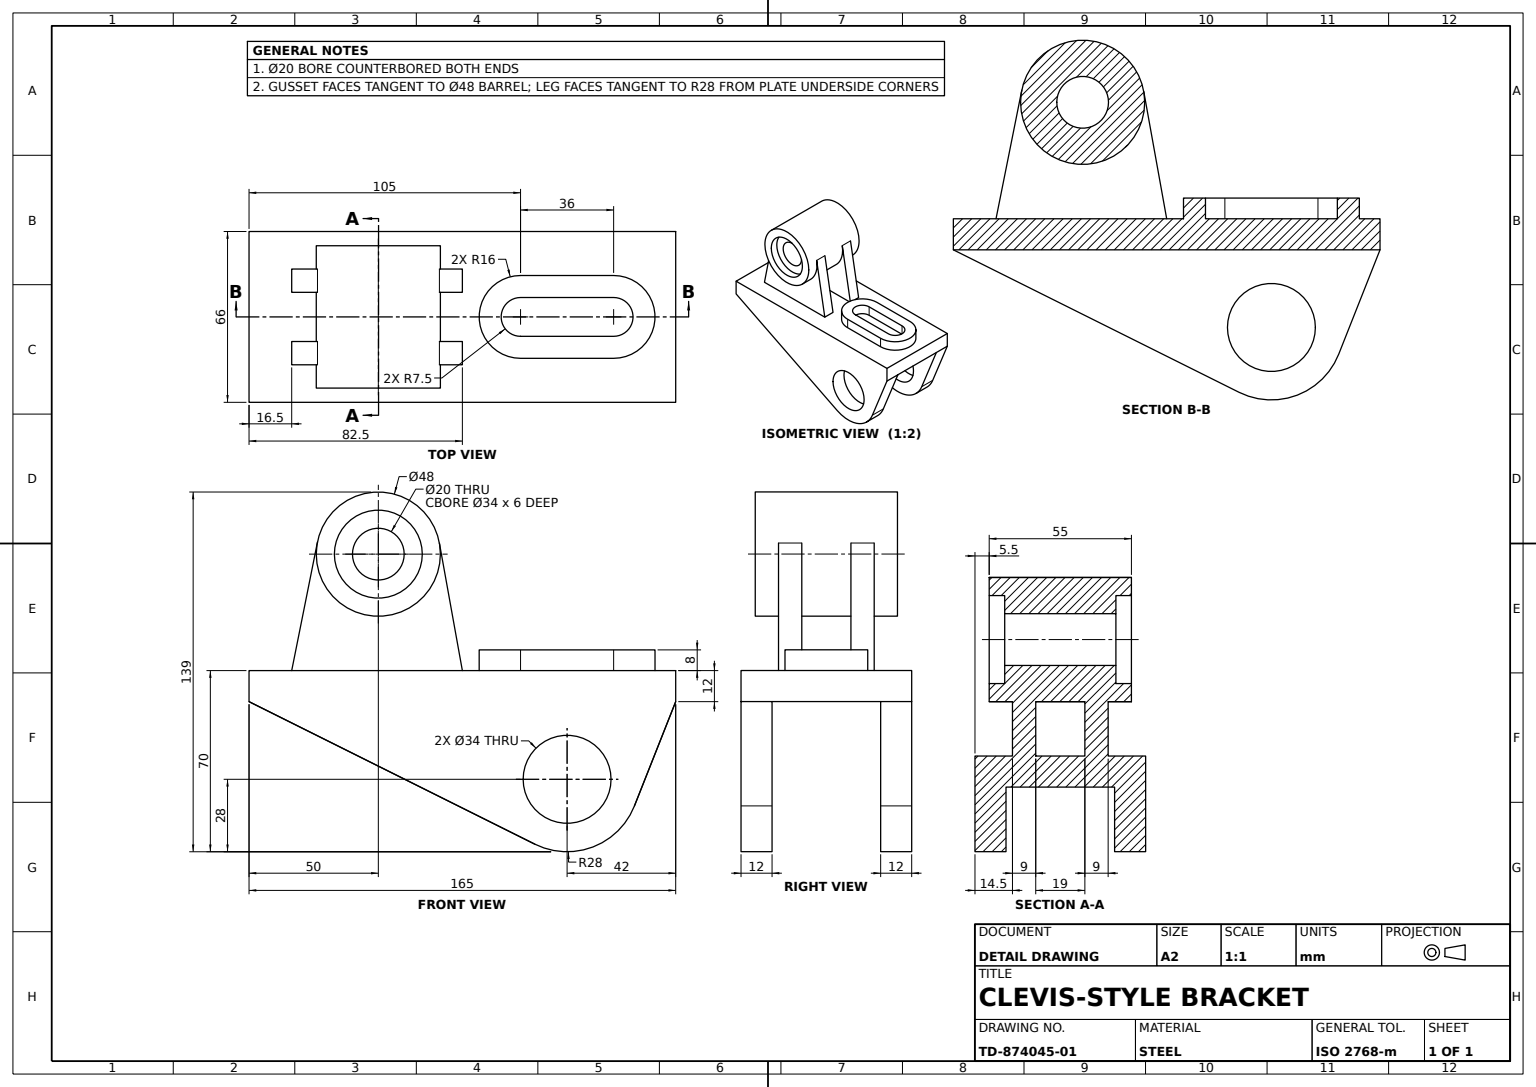
from build123d import *

# Parameters (mm, degrees)
STANCHION_PROFILE_SKETCH_R = 17
STANCHION_BODY_DEPTH       = 33
CORNER_NOTCH_SKETCH_W      = 42
CORNER_NOTCH_SKETCH_H      = 58
CORNER_NOTCH_12X12_DEPTH   = 183.247085025
SLOTTED_BOSS_DEPTH         = 8
HINGE_BARREL_SKETCH_R      = 24
HINGE_BARREL_SKETCH_R_2    = 10
HINGE_BARREL_DEPTH         = 27.5
BARREL_START               = -9
BARREL_GUSSET_DEPTH        = 9
BARREL_RECESS_SKETCH_R     = 17
BARREL_RECESS_CUT_DEPTH    = 6


with BuildPart() as part:
    # Stanchion Profile Sketch → Stanchion Body (new, symmetric)
    with BuildSketch(Plane.XY):
        with BuildLine():
            Line((0, 0), (165, 0))
            Line((165, 0), (165, -12))
            Line((165, -12), (149.032106642, -52.311615965))
            ThreePointArc((149.032106642, -52.311615965), (133.013045842, -68.148401729), (110.513423096, -67.061631974))
            Line((110.513423096, -67.061631974), (0, -12))
            Line((0, -12), (0, 0))
        make_face()
        with Locations((123, -42)):
            Circle(STANCHION_PROFILE_SKETCH_R, mode=Mode.SUBTRACT)
    extrude(amount=STANCHION_BODY_DEPTH, both=True)

    # Corner Notch Sketch → Corner Notch 12x12 (cut, through all)
    with BuildSketch(Plane(origin=(165, 0, 0), x_dir=(0, 0, -1), z_dir=(1, 0, 0))):
        with Locations((0, -41)):
            Rectangle(CORNER_NOTCH_SKETCH_W, CORNER_NOTCH_SKETCH_H)
    extrude(amount=-CORNER_NOTCH_12X12_DEPTH, mode=Mode.SUBTRACT)

    # Slotted Boss Sketch → Slotted Boss (add)
    with BuildSketch(Plane(origin=(0, 0, 0), x_dir=(1, 0, 0), z_dir=(0, 1, 0))):
        with BuildLine():
            Line((105, 16), (141, 16))
            ThreePointArc((141, 16), (157, 0), (141, -16))
            Line((141, -16), (105, -16))
            ThreePointArc((105, -16), (89, 0), (105, 16))
        make_face()
        with BuildLine():
            Line((105, 7.5), (141, 7.5))
            ThreePointArc((141, 7.5), (148.5, 0), (141, -7.5))
            Line((141, -7.5), (105, -7.5))
            ThreePointArc((105, -7.5), (97.5, 0), (105, 7.5))
        make_face(mode=Mode.SUBTRACT)
    extrude(amount=SLOTTED_BOSS_DEPTH)



with BuildPart() as body_2:
    # Hinge Barrel Sketch → Hinge Barrel (new, symmetric)
    with BuildSketch(Plane.XY):
        with Locations((50, 45)):
            Circle(HINGE_BARREL_SKETCH_R)
        with Locations((50, 45)):
            Circle(HINGE_BARREL_SKETCH_R_2, mode=Mode.SUBTRACT)
    extrude(amount=HINGE_BARREL_DEPTH, both=True)


with BuildPart() as part_1:
    add(part.part)

    add(body_2.part)  # Barrel Gusset merges body 2
    # Barrel Gusset Sketch → Barrel Gusset (add)
    with BuildSketch(Plane.XY.offset(27.5).offset(BARREL_START)):
        with BuildLine():
            Line((73.619203331, 49.258313517), (82.5, 0))
            Line((82.5, 0), (16.5, 0))
            Line((16.5, 0), (26.468315489, 49.718031802))
            ThreePointArc((26.468315489, 49.718031802), (49.766012583, 21.001140654), (73.619203331, 49.258313517))
        make_face()
    barrel_gusset = extrude(amount=-BARREL_GUSSET_DEPTH)

    # Barrel Gusset Mirror: Barrel Gusset across plane
    add(barrel_gusset.mirror(Plane.XY))

    # Barrel Recess Sketch → Barrel Recess Cut (cut)
    with BuildSketch(Plane.XY.offset(27.5)):
        with Locations((50, 45)):
            Circle(BARREL_RECESS_SKETCH_R)
    barrel_recess_cut = extrude(amount=-BARREL_RECESS_CUT_DEPTH, mode=Mode.SUBTRACT)

    # Barrel Recess Mirror: Barrel Recess Cut across plane
    add(barrel_recess_cut.mirror(Plane.XY), mode=Mode.SUBTRACT)


solid = part_1.part
